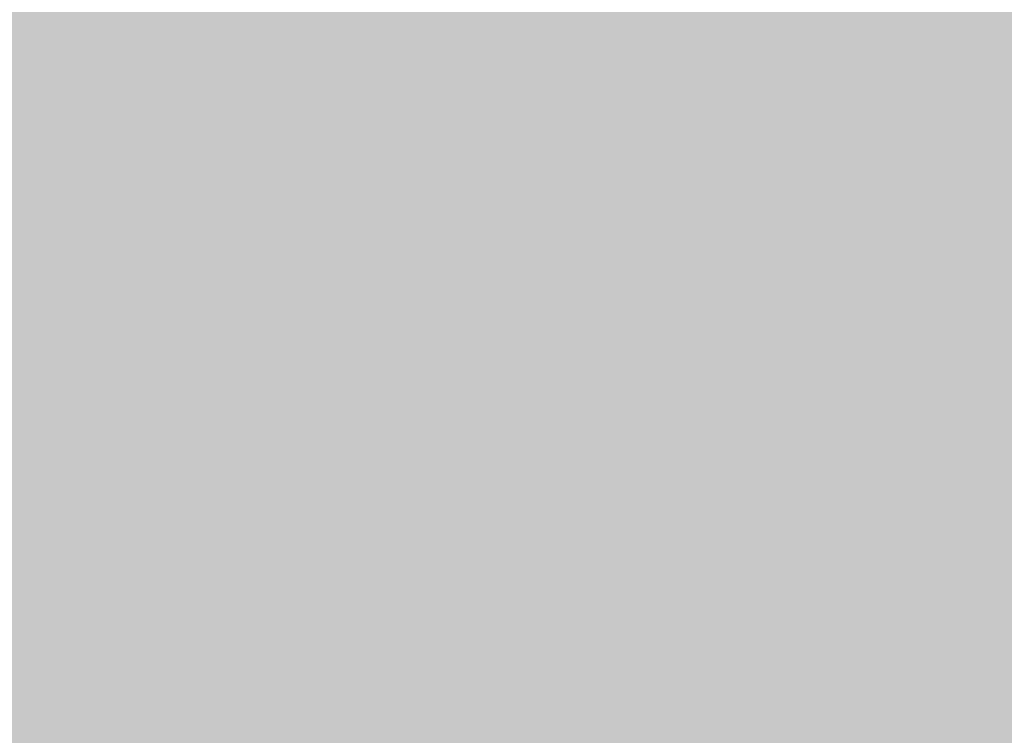
# Model space of a CAD drawing. Units: feet. Extents: x 3168 to 4724, y 827 to 1477.
# Tile 91 of 256: x 3275.224 to 3277.376, y 1096.781 to 1098.344. Entities that reach past the tile are written whole.
import ezdxf

# ---------------------------------------------------------------- set-up
doc = ezdxf.new("R2010")
doc.units = ezdxf.units.FT
doc.layers.add('A-ELEV-PATT', color=8, linetype='Continuous', lineweight=13)

msp = doc.modelspace()

# ---------------------------------------------------------------- hatches: boundary and pattern name
at = {"layer": 'A-ELEV-PATT'}
h = msp.add_hatch(color=256, dxfattribs=at)
h.dxf.hatch_style = 1
edge = h.paths.add_edge_path()
edge.add_ellipse((3552.9058, 979.2201), major_axis=(36.7449, 0), ratio=0.4848485, start_angle=0, end_angle=360)
edge = h.paths.add_edge_path()
edge.add_ellipse((3559.8916, 929.2523), major_axis=(36.7449, 0), ratio=0.4848485, start_angle=0, end_angle=360)
edge = h.paths.add_edge_path()
edge.add_line((3299.3168, 1198.6061), (3479.9167, 1198.6061))
edge.add_line((3479.9167, 1198.6061), (3479.9167, 1209.8686))
edge.add_spline(control_points=[(3479.9167, 1209.8686), (3464.3012, 1209.8686), (3448.6856, 1209.8686), (3410.9491, 1209.8686), (3388.8282, 1209.8686), (3355.6469, 1209.8686), (3344.5864, 1209.8686), (3327.9957, 1209.8686), (3322.4655, 1209.8686), (3314.1702, 1209.8686), (3311.4051, 1209.8686), (3307.2574, 1209.8686), (3305.8748, 1209.8686), (3303.801, 1209.8686), (3303.1097, 1209.8686), (3302.0728, 1209.8686), (3301.7272, 1209.8686), (3301.2087, 1209.8686), (3301.0359, 1209.8686), (3300.7767, 1209.8686), (3300.6903, 1209.8686), (3300.5606, 1209.8686), (3300.5174, 1209.8686), (3300.4526, 1209.8686), (3300.431, 1209.8686), (3300.3986, 1209.8686), (3300.3878, 1209.8686), (3300.3662, 1209.8686), (3300.3457, 1209.8686), (3300.3455, 1209.8686), (3300.3455, 1209.8686), (3300.3433, 1209.8686), (3300.3411, 1209.8686), (3300.3379, 1209.8686), (3300.3368, 1209.8686), (3300.3339, 1209.8686), (3300.3321, 1209.8686), (3300.3255, 1209.8686), (3300.3207, 1209.8686), (3300.3109, 1209.8686), (3300.306, 1209.8686), (3300.2905, 1209.8686), (3300.28, 1209.8686), (3300.2324, 1209.8688), (3300.1953, 1209.869), (3299.9511, 1209.8706), (3299.7448, 1209.8743), (3299.4368, 1209.8833), (3299.3344, 1209.8868), (3299.1811, 1209.8929), (3299.13, 1209.8951), (3298.6522, 1209.9168), (3298.2295, 1209.9457), (3297.6016, 1210.0024), (3297.3934, 1210.0235), (3297.0827, 1210.0583), (3296.9793, 1210.0705), (3296.293, 1210.1549), (3295.7181, 1210.2434), (3294.8687, 1210.3989), (3294.5877, 1210.4545), (3294.1693, 1210.5433), (3294.0304, 1210.5739), (3291.7071, 1211.1012), (3289.6536, 1211.8134), (3285.7763, 1213.564), (3283.9514, 1214.6035), (3280.5122, 1216.9801), (3278.8972, 1218.3176), (3276.3799, 1220.8295), (3275.416, 1221.9177), (3274.0393, 1223.7077), (3273.581, 1224.3495), (3273.1432, 1225.0163)], knot_values=[39.119033, 39.119033, 39.119033, 39.119033, 39.286353, 39.286353, 39.523379, 39.523379, 39.641892, 39.641892, 39.701148, 39.701148, 39.730777, 39.730777, 39.745591, 39.745591, 39.752998, 39.752998, 39.756701, 39.756701, 39.758553, 39.758553, 39.759479, 39.759479, 39.759942, 39.759942, 39.760173, 39.760173, 39.760289, 39.760289, 39.760405, 39.760405, 39.760463, 39.760463, 39.763389, 39.763389, 39.764851, 39.764851, 39.767304, 39.767304, 39.773825, 39.773825, 39.78057, 39.78057, 39.79477, 39.79477, 39.845194, 39.845194, 40.126715, 40.126715, 40.267476, 40.267476, 40.337856, 40.337856, 40.927023, 40.927023, 41.221606, 41.221606, 41.368898, 41.368898, 42.202622, 42.202622, 42.619485, 42.619485, 42.827916, 42.827916, 46.118323, 46.118323, 49.408731, 49.408731, 52.699139, 52.699139, 54.927489, 54.927489, 56.104228, 56.104228, 56.104228, 56.104228], weights=[1, 1, 1, 1, 1, 1, 1, 1, 1, 1, 1, 1, 1, 1, 1, 1, 1, 1, 1, 1, 1, 1, 1, 1, 1, 1, 1, 1, 1, 1, 1, 1, 1, 1, 1, 1, 1, 1, 1, 1, 1, 1, 1, 1, 1, 1, 1, 1, 1, 1, 1, 1, 1, 1, 1, 1, 1, 1, 1, 1, 1, 1, 1, 1, 1, 1, 1, 1, 1, 1, 1, 1, 1, 1], degree=3, periodic=0)
edge.add_line((3273.1432, 1225.0163), (3273.1432, 1099.0163))
edge.add_line((3273.1432, 1099.0163), (3299.3168, 1099.0163))
edge.add_line((3299.3168, 1099.0163), (3299.3168, 1198.6061))
edge = h.paths.add_edge_path()
edge.add_line((3304.7584, 1324.1581), (3479.9167, 1324.1581))
edge.add_line((3479.9167, 1324.1581), (3479.9167, 1335.7146))
edge.add_line((3479.9167, 1335.7146), (3269.1616, 1335.7146))
edge.add_spline(control_points=[(3269.1616, 1335.7146), (3264.0242, 1335.7146), (3258.3641, 1328.9582), (3259.2643, 1323.9003)], knot_values=[0, 0, 0, 0, 15.412191, 15.412191, 15.412191, 15.412191], degree=3, periodic=0)
edge.add_line((3259.2643, 1323.9003), (3265.5168, 1288.7691))
edge.add_line((3265.5168, 1288.7691), (3275.2651, 1261.5456))
edge.add_line((3275.2651, 1261.5456), (3304.7584, 1261.5456))
edge.add_line((3304.7584, 1261.5456), (3304.7584, 1324.1581))
h = msp.add_hatch(color=256, dxfattribs=at)
h.dxf.hatch_style = 1
h.paths.add_polyline_path([(3384.5252, 1099.0163), (3335.0292, 1099.0163), (3299.3168, 1099.0163), (3273.1432, 1099.0163), (3217.5654, 1099.0163), (3168.0693, 827.1163), (3335.0292, 827.1163)])

doc.saveas('drawing.dxf')
